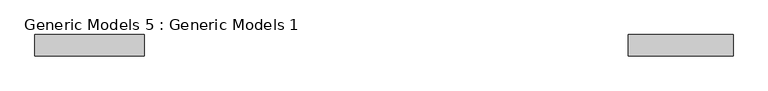
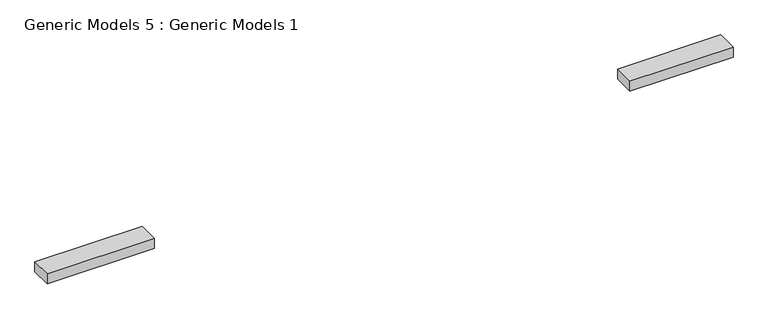
"""IFC4 building model written with IfcOpenShell, lengths in millimetres: proxy geometry, Generic Models 5 : Generic Models 1."""

from ifc_helpers import new_model, si_unit, frame, origin, place, context, project, spatial, polyline, outline, extrude, source, transform, mapped, element, save


def generic_models_5_generic_models_1_03e322a7(model_context):
    return source(origin(), model_context, "Body", "SweptSolid", [
        extrude(outline(polyline([(-4635.1670283, -6837.0727897), (-6122.6771954, -6837.0727897), (-6122.6771954, -6532.2727897), (-4635.1670283, -6532.2727897), (-4635.1670283, -6837.0727897)])), frame((0.0, 0.0, 5613.4), z_axis=(0.0, 0.0, 1.0), x_axis=(1.0, 0.0, 0.0)), (0.0, 0.0, 1.0), 152.4),
        extrude(outline(polyline([(-12974.453029, -6837.0727897), (-14521.3088608, -6837.0727897), (-14521.3088608, -6532.2727897), (-12974.453029, -6532.2727897), (-12974.453029, -6837.0727897)])), frame((0.0, 0.0, 5613.4), z_axis=(0.0, 0.0, 1.0), x_axis=(1.0, 0.0, 0.0)), (0.0, 0.0, 1.0), 152.4),
    ])


if __name__ == "__main__":
    model = new_model("IFC4")
    model_context = context("Model", 3, world=origin())
    ifc_project = project(units=[si_unit("LENGTHUNIT", "METRE", prefix="MILLI")], contexts=[model_context])
    site = spatial("IfcSite", under=ifc_project)
    building = spatial("IfcBuilding", under=site)
    placement = place(None, origin())
    generic_models_5_generic_models_1_shape = generic_models_5_generic_models_1_03e322a7(model_context)
    element("IfcBuildingElementProxy", 1, Name="Generic Models 5 : Generic Models 1", ObjectType="Generic Models 5 : Generic Models 1", at=placement, inside=building, context=model_context, shape_type="MappedRepresentation", body=[
        mapped(generic_models_5_generic_models_1_shape, transform((0.0, 0.0, 0.0), x_axis=(1.0, 0.0, 0.0), y_axis=(0.0, 1.0, 0.0), z_axis=(0.0, 0.0, 1.0))),
    ])
    save(model, "model.ifc")
